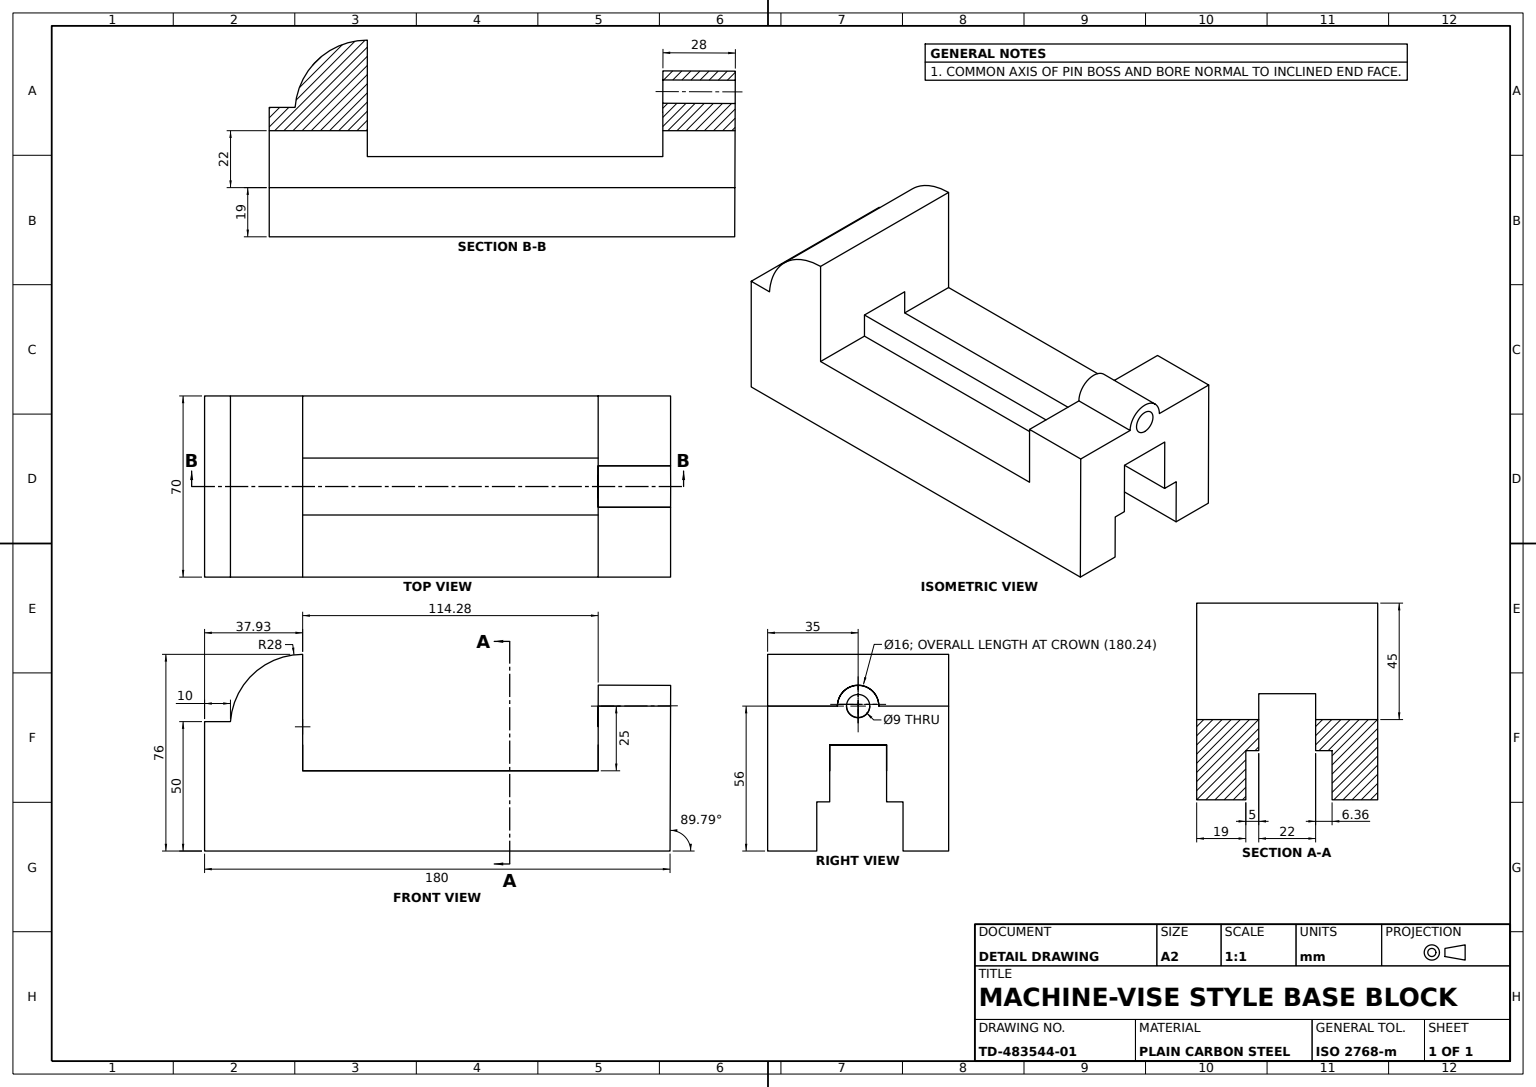
from build123d import *

# Parameters (mm, degrees)
BASE_BODY_DEPTH    = 70
PIN_BOSS_SKETCH_R  = 8
PIN_BOSS_DEPTH     = 28
PIN_HOLE_SKETCH_R  = 4.5
PIN_HOLE_DEPTH     = 28
END_SLOT_CUT_DEPTH = 208.754707688


with BuildPart() as part:
    # Base Profile Sketch → Base Body (new body)
    with BuildSketch(Plane.XY):
        with BuildLine():
            Line((0, 0), (180, 0))
            Line((180, 0), (180.209078325, 55.999609697))
            Line((180.209078325, 55.999609697), (152.209078325, 55.999609697))
            Line((152.209078325, 55.999609697), (152.209078325, 30.999609697))
            Line((152.209078325, 30.999609697), (37.928452135, 30.999609697))
            Line((37.928452135, 30.999609697), (37.928452135, 75.999609697))
            ThreePointArc((37.928452135, 75.999609697), (18.849811309, 68.493644543), (10, 50))
            Line((10, 50), (0, 50))
            Line((0, 50), (0, 0))
        make_face()
    extrude(amount=-BASE_BODY_DEPTH)

    # Pin Boss Sketch → Pin Boss (add)
    with BuildSketch(Plane(origin=(179.99749092, -0.67203279, 0), x_dir=(0, 0, -1), z_dir=(0.9999930303095579, -0.0037335415234940133, 0))):
        with Locations(Location((35, 56.672037474, 0), (0, 0, 90))):
            Circle(PIN_BOSS_SKETCH_R)
    extrude(amount=-PIN_BOSS_DEPTH)

    # Pin Hole Sketch → Pin Hole (cut)
    with BuildSketch(Plane(origin=(179.99749092, -0.67203279, 0), x_dir=(0, 0, -1), z_dir=(0.9999930303095579, -0.0037335415234940133, 0))):
        with Locations(Location((35, 56.672037474, 0), (0, 0, 90))):
            Circle(PIN_HOLE_SKETCH_R)
    extrude(amount=-PIN_HOLE_DEPTH, mode=Mode.SUBTRACT)

    # End Slot Sketch → End Slot Cut (cut, through all)
    with BuildSketch(Plane.ZY):
        Polygon((-52.359197148, 0), (-52.359197148, 19), (-46, 19), (-46, 41), (-24, 41), (-24, 19), (-19, 19), (-19, 0), align=None)
    extrude(amount=-END_SLOT_CUT_DEPTH, mode=Mode.SUBTRACT)


solid = part.part
